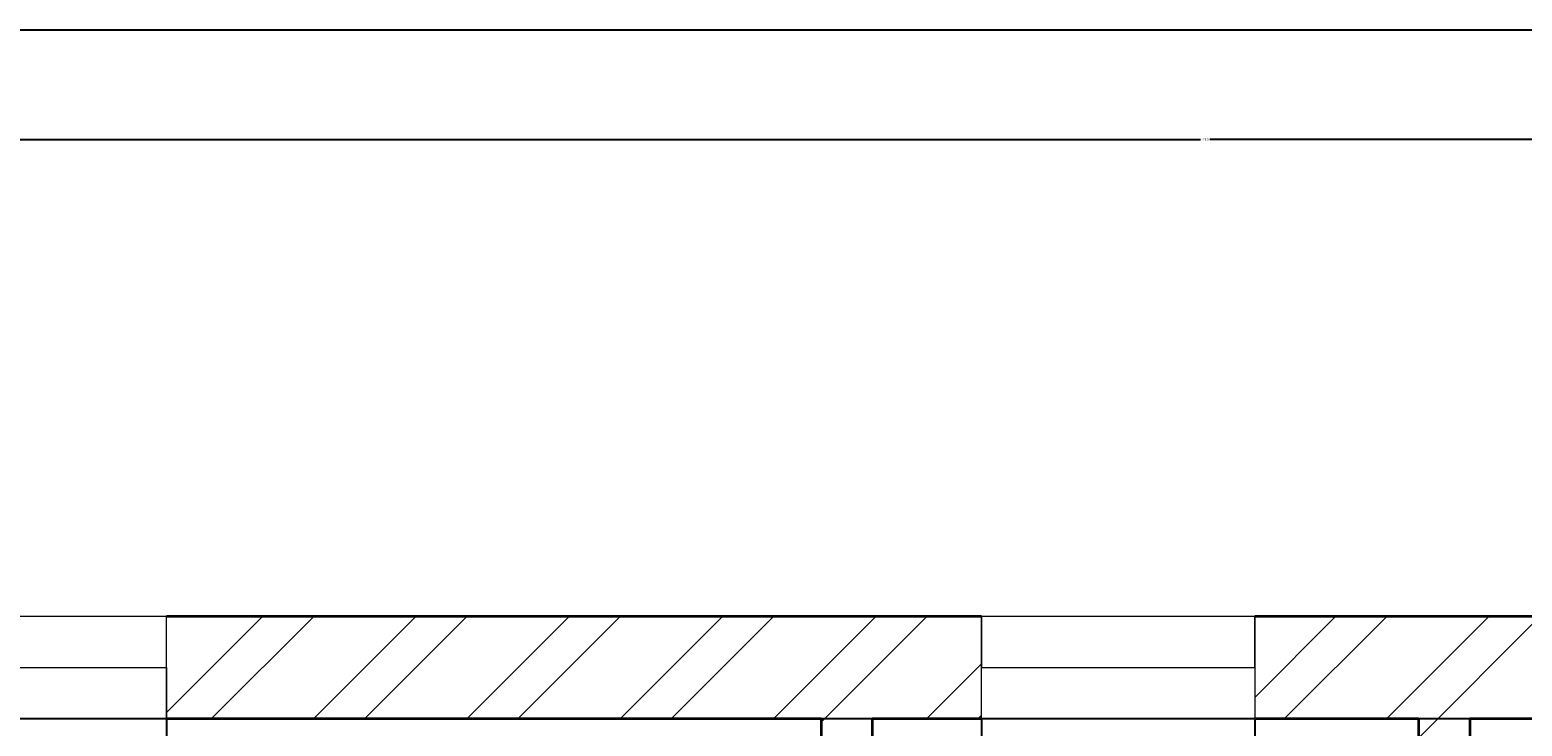
# Model space of a CAD drawing. Units: inches. Extents: x 1748 to 2382, y 1346 to 2284.
# Tile 24 of 26: x 1956 to 2088, y 2223 to 2284. Entities that reach past the tile are written whole.
import ezdxf

# ---------------------------------------------------------------- set-up
doc = ezdxf.new("R2010")
doc.units = ezdxf.units.IN
for name, color, linetype, lineweight in [('A-ANNO-DIMS', 2, 'Continuous', 18), ('A-ANNO-TTLB', 7, 'Continuous', 25), ('A-GLAZ', 191, 'Continuous', 18), ('A-WALL', 7, 'Continuous', 35), ('A-WALL-PATT', 9, 'Continuous', 13)]:
    doc.layers.add(name, color=color, linetype=linetype, lineweight=lineweight)
doc.styles.get("Standard").update_dxf_attribs({"font": 'arial.ttf'})
doc.dimstyles.get("Standard").update_dxf_attribs({"dimtxt": 0.18, "dimasz": 0.18, "dimexe": 0.18, "dimexo": 0.0625, "dimgap": 0.09, "dimtad": 0, "dimtih": 1, "dimtoh": 1, "dimdec": 4, "dimzin": 0, "dimdsep": 46, "dimtxsty": 'Standard', "dimcen": 0.09, "dimadec": 0, "dimazin": 0, "dimtfac": 1, "dimtdec": 4, "dimtofl": 0, "dimtmove": 0, "dimatfit": 3, "dimfxl": 1, "dimtolj": 1, "dimtzin": 0, "dimarcsym": 0})

# ---------------------------------------------------------------- blocks, each defined once
blk = doc.blocks.new('WIN-60-DEEP')
for p, q in [((0, 9), (0, 0)), ((60, 9), (0, 9)), ((60, 4.5), (60, 9)), ((60, 9), (60, 0)), ((0, 0), (0, 4.5)), ((0, 4.5), (60, 4.5)), ((0, 0), (60, 0))]:
    blk.add_line(p, q)
blk = doc.blocks.new('*D34')
at = {"layer": 'A-ANNO-DIMS', "color": 0, "lineweight": -2, "transparency": 16777216}
for p, q in [((1821.96, 2232.91), (1821.96, 2274.93)), ((1822.14, 2274.75), (2059.31, 2274.75)), ((2297.28, 2274.75), (2060.11, 2274.75)), ((2297.46, 2232.91), (2297.46, 2274.93))]:
    blk.add_line(p, q, dxfattribs=at)
at = {"layer": 'A-ANNO-DIMS', "color": 0, "transparency": 16777216}
for points in [[(1822.14, 2274.78), (1822.14, 2274.72), (1821.96, 2274.75)], [(2297.28, 2274.78), (2297.28, 2274.72), (2297.46, 2274.75)]]:
    blk.add_solid(points, dxfattribs=at)
at = {"layer": 'Defpoints', "color": 0, "transparency": 16777216}
for p in [(2297.46, 2274.75), (1821.96, 2232.85), (2297.46, 2232.85)]:
    blk.add_point(p, dxfattribs=at)
at = {"layer": 'A-ANNO-DIMS', "color": 0, "transparency": 16777216, "insert": (2059.71, 2274.75), "char_height": 0.18, "attachment_point": 5}
blk.add_mtext('\\A1;475.5', dxfattribs=at)
blk = doc.blocks.new('*D51')
at = {"layer": 'A-ANNO-DIMS', "color": 0, "lineweight": -2, "transparency": 16777216}
for p, q in [((1968.44, 2223.79), (1968.44, 1360.47)), ((2040.07, 2223.79), (2040.07, 1360.47)), ((1968.62, 1360.65), (2003.86, 1360.65)), ((2039.89, 1360.65), (2004.65, 1360.65))]:
    blk.add_line(p, q, dxfattribs=at)
at = {"layer": 'A-ANNO-DIMS', "color": 0, "transparency": 16777216}
for points in [[(1968.62, 1360.68), (1968.62, 1360.62), (1968.44, 1360.65)], [(2039.89, 1360.68), (2039.89, 1360.62), (2040.07, 1360.65)]]:
    blk.add_solid(points, dxfattribs=at)
at = {"layer": 'Defpoints', "color": 0, "transparency": 16777216}
for p in [(1968.44, 2223.85), (2040.07, 2223.85), (2040.07, 1360.65)]:
    blk.add_point(p, dxfattribs=at)
at = {"layer": 'A-ANNO-DIMS', "color": 0, "transparency": 16777216, "insert": (2004.26, 1360.65), "char_height": 0.18, "attachment_point": 5}
blk.add_mtext('\\A1;71.62', dxfattribs=at)
blk = doc.blocks.new('*D52')
at = {"layer": 'A-ANNO-DIMS', "color": 0, "lineweight": -2, "transparency": 16777216}
for p, q in [((2064.07, 2223.79), (2064.07, 1360.47)), ((2091.4, 2223.79), (2091.4, 1360.47)), ((2064.25, 1360.65), (2077.34, 1360.65)), ((2091.22, 1360.65), (2078.13, 1360.65))]:
    blk.add_line(p, q, dxfattribs=at)
at = {"layer": 'A-ANNO-DIMS', "color": 0, "transparency": 16777216}
for points in [[(2064.25, 1360.68), (2064.25, 1360.62), (2064.07, 1360.65)], [(2091.22, 1360.68), (2091.22, 1360.62), (2091.4, 1360.65)]]:
    blk.add_solid(points, dxfattribs=at)
at = {"layer": 'Defpoints', "color": 0, "transparency": 16777216}
for p in [(2064.07, 2223.85), (2091.4, 2223.85), (2091.4, 1360.65)]:
    blk.add_point(p, dxfattribs=at)
at = {"layer": 'A-ANNO-DIMS', "color": 0, "transparency": 16777216, "insert": (2077.73, 1360.65), "char_height": 0.18, "attachment_point": 5}
blk.add_mtext('\\A1;27.33', dxfattribs=at)
blk = doc.blocks.new('*D68')
at = {"layer": 'A-ANNO-DIMS', "color": 0, "lineweight": -2, "transparency": 16777216}
for p, q in [((1865.52, 2223.85), (2339.54, 2223.85)), ((2339.36, 2223.67), (2339.36, 2217.07)), ((2339.36, 2210.1), (2339.36, 2216.7)), ((1865.52, 2209.92), (2339.54, 2209.92))]:
    blk.add_line(p, q, dxfattribs=at)
at = {"layer": 'A-ANNO-DIMS', "color": 0, "transparency": 16777216}
for points in [[(2339.33, 2223.67), (2339.39, 2223.67), (2339.36, 2223.85)], [(2339.33, 2210.1), (2339.39, 2210.1), (2339.36, 2209.92)]]:
    blk.add_solid(points, dxfattribs=at)
at = {"layer": 'Defpoints', "color": 0, "transparency": 16777216}
for p in [(1865.46, 2223.85), (2339.36, 2223.85), (1865.46, 2209.92)]:
    blk.add_point(p, dxfattribs=at)
at = {"layer": 'A-ANNO-DIMS', "color": 0, "transparency": 16777216, "insert": (2339.36, 2216.88), "char_height": 0.18, "attachment_point": 5}
blk.add_mtext('\\A1;13.93', dxfattribs=at)

msp = doc.modelspace()

# ---------------------------------------------------------------- hatches: boundary and pattern name
at = {"layer": 'A-WALL-PATT'}
h = msp.add_hatch(dxfattribs=at)
h.set_pattern_fill('ANSI32', color=256)
h.paths.add_polyline_path([(1908.4445, 2232.8497), (1821.9607, 2232.8497), (1821.9607, 2223.8497), (1865.4607, 2223.8497), (1865.4607, 2209.9185), (1869.9607, 2209.9185), (1869.9607, 2223.8497), (1908.4445, 2223.8497), (1908.4445, 2228.3497)])
h.paths.add_polyline_path([(2040.0683, 2232.8497), (1968.4445, 2232.8497), (1968.4445, 2223.8497), (2025.9607, 2223.8497), (2025.9607, 2130.3497), (2032.1341, 2130.3497), (2032.1341, 2132.5997), (2032.1341, 2134.8497), (2030.4607, 2134.8497), (2030.4607, 2223.8497), (2040.0683, 2223.8497)])
h.paths.add_polyline_path([(2091.3969, 2232.8497), (2064.0683, 2232.8497), (2064.0683, 2223.8497), (2078.4607, 2223.8497), (2078.4607, 2134.8497), (2051.1563, 2134.8497), (2051.1563, 2130.3497), (2078.4607, 2130.3497), (2078.4607, 2128.6813), (2082.9607, 2128.6813), (2082.9607, 2130.3497), (2086.1879, 2130.3497), (2086.1879, 2132.5997), (2086.1879, 2134.8497), (2082.9607, 2134.8497), (2082.9607, 2223.8497), (2091.3969, 2223.8497), (2091.3969, 2228.3497)])
h.paths.add_polyline_path([(2167.0164, 2232.8497), (2115.3969, 2232.8497), (2115.3969, 2223.8497), (2130.9607, 2223.8497), (2130.9607, 2134.8497), (2106.9607, 2134.8497), (2106.9607, 2130.3497), (2135.4607, 2130.3497), (2135.4607, 2223.8497), (2167.0164, 2223.8497), (2167.0164, 2228.3497)])
h.paths.add_polyline_path([(1869.9607, 2149.9185), (1865.4607, 2149.9185), (1865.4607, 2127.8942), (1869.9607, 2127.8942)])
h.paths.add_polyline_path([(2082.9607, 2104.4871), (2080.7107, 2104.4871), (2078.4607, 2104.4871), (2078.4607, 2103.8497), (1869.9607, 2103.8497), (1869.9607, 2108.6062), (1867.7107, 2108.6062), (1865.4607, 2108.6062), (1865.4607, 2103.8497), (1821.9607, 2103.8497), (1821.9607, 2099.3497), (1865.4607, 2099.3497), (1865.4607, 2094.7509), (1869.9607, 2094.7509), (1869.9607, 2099.3497), (2025.9607, 2099.3497), (2025.9607, 2096.4326), (2030.4607, 2096.4326), (2030.4607, 2099.3497), (2082.9607, 2099.3497)])
h.paths.add_polyline_path([(1928.9457, 1401.1212), (2176.8693, 1401.1212), (2176.8693, 1438.214), (1928.9457, 1438.214)], flags=9)
h.paths.add_polyline_path([(2122.2668, 2048.1927), (2177.9387, 2048.1927), (2177.9387, 2066.85), (2122.2668, 2066.85)], flags=9)
h.paths.add_polyline_path([(2272.688, 2153.8197), (2272.688, 2216.746), (2262.3845, 2216.746), (2262.3845, 2153.8197)], flags=9)
h.paths.add_polyline_path([(2157.2928, 2166.5593), (2196.3822, 2166.5593), (2196.3822, 2185.2167), (2157.2928, 2185.2167)], flags=9)
h.paths.add_polyline_path([(2089.3407, 2162.0698), (2124.3987, 2162.0698), (2124.3987, 2180.7272), (2089.3407, 2180.7272)], flags=9)
h.paths.add_polyline_path([(2037.4521, 2160.0913), (2072.5101, 2160.0913), (2072.5101, 2178.7486), (2037.4521, 2178.7486)], flags=9)
h.paths.add_polyline_path([(1884.7894, 2104.1554), (1923.6297, 2104.1554), (1923.6297, 2122.8127), (1884.7894, 2122.8127)], flags=9)
h.paths.add_polyline_path([(1851.2832, 2142.9749), (1851.2832, 2199.3051), (1840.9796, 2199.3051), (1840.9796, 2142.9749)], flags=9)
h.paths.add_polyline_path([(1844.8763, 2017.2834), (1844.8763, 2073.6136), (1834.5728, 2073.6136), (1834.5728, 2017.2834)], flags=9)
h.paths.add_polyline_path([(1897.1577, 2073.1279), (1935.9981, 2073.1279), (1935.9981, 2091.7853), (1897.1577, 2091.7853)], flags=9)
h.paths.add_polyline_path([(1952.3395, 1802.4231), (2008.0114, 1802.4231), (2008.0114, 1821.0805), (1952.3395, 1821.0805)], flags=9)
h.paths.add_polyline_path([(1978.8184, 1857.6841), (2017.7338, 1857.6841), (2017.7338, 1876.3415), (1978.8184, 1876.3415)], flags=9)
h.paths.add_polyline_path([(1979.6513, 1925.9516), (2008.8089, 1925.9516), (2008.8089, 1944.6089), (1979.6513, 1944.6089)], flags=9)
h.paths.add_polyline_path([(1838.5553, 1860.3527), (1877.3957, 1860.3527), (1877.3957, 1879.01), (1838.5553, 1879.01)], flags=9)
h.paths.add_polyline_path([(1883.9018, 1787.3013), (1883.9018, 1843.6315), (1873.5983, 1843.6315), (1873.5983, 1787.3013)], flags=9)
h.paths.add_polyline_path([(1873.7079, 1509.1938), (1873.7079, 1583.7709), (1863.4044, 1583.7709), (1863.4044, 1509.1938)], flags=9)
h.paths.add_polyline_path([(1916.2259, 1603.3681), (1955.0663, 1603.3681), (1955.0663, 1622.0254), (1916.2259, 1622.0254)], flags=9)
h.paths.add_polyline_path([(1876.3013, 1636.757), (1876.3013, 1693.0871), (1865.9978, 1693.0871), (1865.9978, 1636.757)], flags=9)
h.paths.add_polyline_path([(1921.3138, 1521.8316), (1964.0662, 1521.8316), (1964.0662, 1540.489), (1921.3138, 1540.489)], flags=9)
h.paths.add_polyline_path([(2017.5657, 1497.5078), (2046.7983, 1497.5078), (2046.7983, 1516.1651), (2017.5657, 1516.1651)], flags=9)
h.paths.add_polyline_path([(2066.8661, 1499.3902), (2096.0988, 1499.3902), (2096.0988, 1518.0475), (2066.8661, 1518.0475)], flags=9)
h.paths.add_polyline_path([(2155.4835, 1571.6596), (2198.2358, 1571.6596), (2198.2358, 1590.3169), (2155.4835, 1590.3169)], flags=9)
h.paths.add_polyline_path([(2094.9136, 1664.6812), (2150.5855, 1664.6812), (2150.5855, 1683.3386), (2094.9136, 1683.3386)], flags=9)
h.paths.add_polyline_path([(2257.6902, 1863.1628), (2269.8935, 1863.1628), (2269.8935, 1873.4664), (2257.6902, 1873.4664)], flags=9)
h.paths.add_polyline_path([(2164.0748, 1880.3089), (2189.8694, 1880.3089), (2189.8694, 1890.6124), (2164.0748, 1890.6124)], flags=9)
h.paths.add_polyline_path([(2239.4394, 1931.0585), (2268.8187, 1931.0585), (2268.8187, 1949.7159), (2239.4394, 1949.7159)], flags=9)

# ---------------------------------------------------------------- linework, layer by layer
at = {"layer": 'A-ANNO-TTLB'}
msp.add_lwpolyline([(1747.8112, 2284.3704), (2382.1361, 2284.3704), (2382.1361, 1346.4899), (1747.8112, 1346.4899)], close=True, dxfattribs=at)
at = {"layer": 'A-GLAZ'}
for p, q in [((2040.0683, 2223.8497), (2040.0683, 2232.8497)), ((2040.0683, 2232.8497), (2040.0683, 2228.3497)), ((2040.0683, 2232.8497), (2064.0683, 2232.8497)), ((2064.0683, 2228.3497), (2064.0683, 2232.8497)), ((2064.0683, 2232.8497), (2064.0683, 2223.8497)), ((2040.0683, 2228.3497), (2064.0683, 2228.3497)), ((2064.0683, 2223.8497), (2040.0683, 2223.8497))]:
    msp.add_line(p, q, dxfattribs=at)
at = {"layer": 'A-WALL'}
for p, q in [((1968.4445, 2232.8497), (2040.0683, 2232.8497)), ((2064.0683, 2232.8497), (2091.3969, 2232.8497)), ((1968.4445, 2223.8497), (2025.9607, 2223.8497)), ((2025.9607, 2223.8497), (2025.9607, 2130.3497)), ((2030.4607, 2223.8497), (2030.4607, 2134.8497)), ((2030.4607, 2223.8497), (2040.0683, 2223.8497)), ((2064.0683, 2223.8497), (2078.4607, 2223.8497)), ((2078.4607, 2223.8497), (2078.4607, 2134.8497)), ((2082.9607, 2223.8497), (2082.9607, 2134.8497)), ((2082.9607, 2223.8497), (2091.3969, 2223.8497))]:
    msp.add_line(p, q, dxfattribs=at)

# ---------------------------------------------------------------- block references
at = {"layer": 'A-GLAZ', "extrusion": (0, 0, -1), "zscale": -1, "rotation": 180}
msp.add_blockref('WIN-60-DEEP', (-1908.444, 2232.8493), dxfattribs=at)

# ---------------------------------------------------------------- dimensions: what is measured, and where the dimension line sits
at = {"layer": 'A-ANNO-DIMS'}
for base, p1, p2, override, picture, middle in [((2297.4607, 2274.7497), (1821.9607, 2232.8497), (2297.4607, 2232.8497), {"dimdec": 1, "dimlfac": 1, "dimrnd": 0, "dimzin": 0, "dimdsep": 46, "dimlunit": 2}, '*D34', (2059.7107, 2274.7497)), ((2040.0683, 1360.6451), (1968.4445, 2223.8497), (2040.0683, 2223.8497), {"dimdec": 2, "dimlfac": 1, "dimrnd": 0, "dimzin": 0, "dimdsep": 46, "dimlunit": 2}, '*D51', (2004.2564, 1360.6451)), ((2091.3969, 1360.6451), (2064.0683, 2223.8497), (2091.3969, 2223.8497), {"dimdec": 2, "dimlfac": 1, "dimrnd": 0, "dimzin": 0, "dimdsep": 46, "dimlunit": 2}, '*D52', (2077.7326, 1360.6451))]:
    dim = msp.add_linear_dim(base=base, p1=p1, p2=p2, dimstyle='Standard', override=override, dxfattribs=at)
    dim.commit()
    dim.dimension.update_dxf_attribs({"geometry": picture, "text_midpoint": middle})
dim = msp.add_linear_dim(base=(2339.3607, 2223.8497), p1=(1865.4607, 2209.9185), p2=(1865.4607, 2223.8497), angle=90, dimstyle='Standard', override={"dimdec": 2, "dimlfac": 1, "dimrnd": 0, "dimzin": 0, "dimdsep": 46, "dimlunit": 2}, dxfattribs=at)
dim.commit()
dim.dimension.update_dxf_attribs({"geometry": '*D68', "text_midpoint": (2339.3607, 2216.8841)})

doc.saveas('drawing.dxf')
